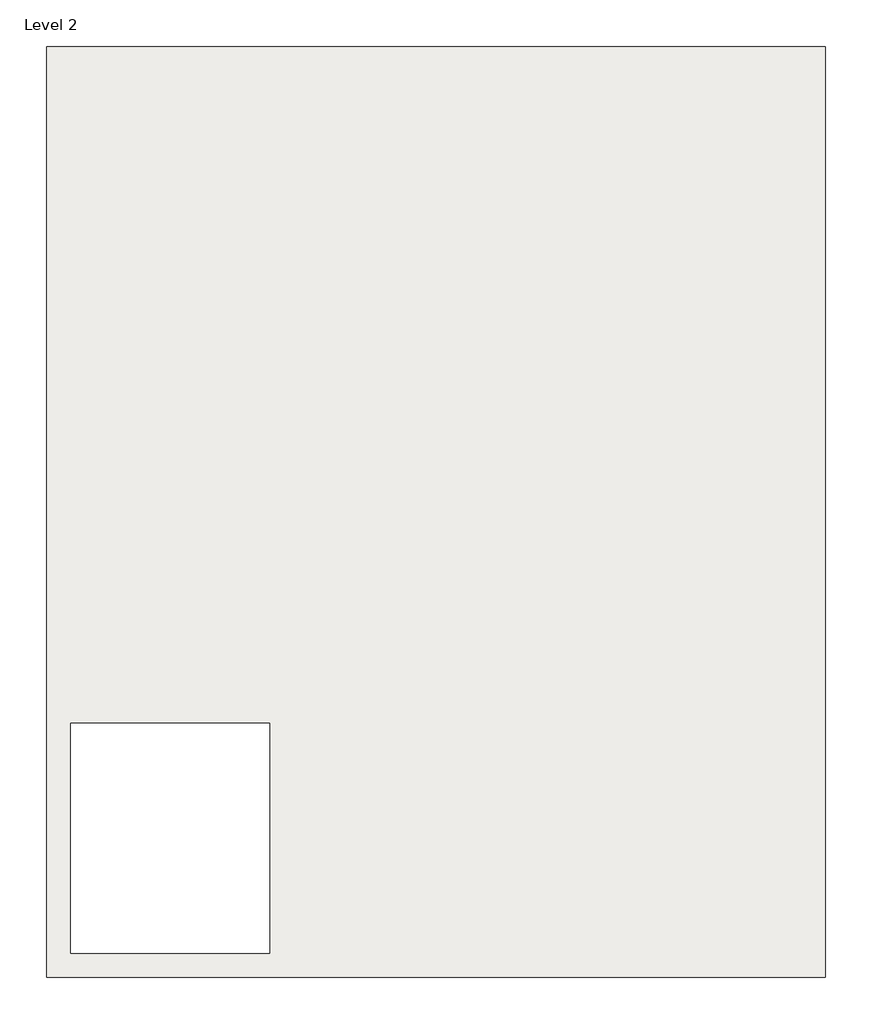
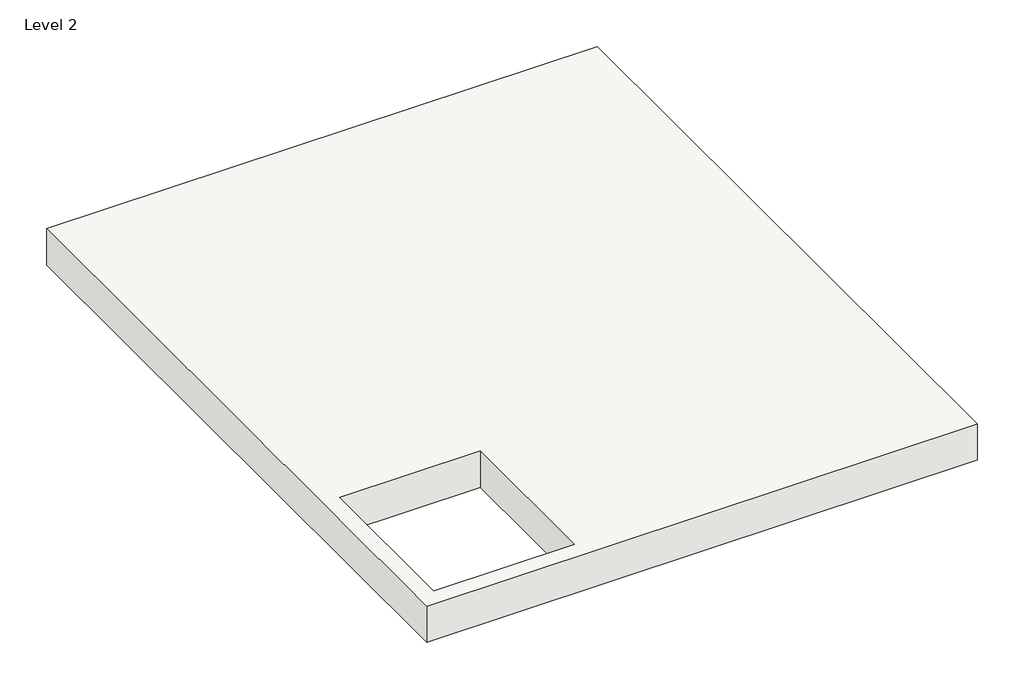
# One storey: 1 roof.
"""IFC4 building model written with IfcOpenShell, lengths in millimetres."""

from ifc_helpers import new_model, si_unit, frame, origin, place, context, project, spatial, polyline, outline, extrude, element, save

model = new_model("IFC4")

# Units and contexts
model_context = context("Model", 3, world=origin())
ifc_project = project(units=[si_unit("LENGTHUNIT", "METRE", prefix="MILLI")], contexts=[model_context])

# Site, building, storey
site = spatial("IfcSite", under=ifc_project)
building = spatial("IfcBuilding", under=site)
storey = spatial("IfcBuildingStorey", under=building, Name="Level 2", Elevation=3048.0)

# Roof
placement = place(None, origin())
element("IfcRoof", 1, ObjectType="Steel Truss - Insulation on Metal Deck - EPDM", at=placement, inside=storey, context=model_context, shape_type="SweptSolid", body=[
    extrude(outline(polyline([(-10104.282173, 13557.9549175), (-2281.082173, 13557.9549175), (-2281.082173, 4210.7549175), (-10104.282173, 4210.7549175), (-10104.282173, 13557.9549175)]), holes=[polyline([(-9863.5624692, 4453.0466042), (-7865.5311534, 4453.0466042), (-7865.5311534, 6764.4466042), (-9863.5624692, 6764.4466042), (-9863.5624692, 4453.0466042)])]), frame((0.0, 0.0, 3048.0), z_axis=(0.0, 0.0, 1.0), x_axis=(1.0, 0.0, 0.0)), (0.0, 0.0, 1.0), 546.1),
])

save(model, "model.ifc")

# Revit data of these elements
# Type "Steel Truss - Insulation on Metal Deck - EPDM"
#   Assembly Code = "B1020"
#   Layers, outside or top first: 0' - 0 1/4" "Roofing, EPDM Membrane" (function 4); 0' - 5" "Rigid insulation" (function 3); 0' - 0 1/4" "Metal Deck" (function 1); 1' - 4" "Structure, Steel Bar Joist Layer" (function 1)
# Element 1 (IfcRoof, "Steel Truss - Insulation on Metal Deck - EPDM")
#   built-in parameter 1001705 = 11.7917 (stored number, unit not read)
#   built-in parameter 1001710 = 33615
#   Phase Created = New Construction
#   Materials on its faces: "Structure, Steel Bar Joist Layer", "Roofing, EPDM Membrane"
# Materials
#   "Roofing, EPDM Membrane": class "Generic", colour RGB 127 127 127, transparency 0, Description = "EPDM roof membrane", Cost = 0
#   "Rigid insulation": class "Generic", colour RGB 127 127 127, transparency 0, Description = "Rigid foam insulation board", Cost = 0
#   "Metal Deck": class "Metal", colour RGB 199 199 199, transparency 0, Description = "Steel, mill finish", Cost = 0
#   "Structure, Steel Bar Joist Layer": class "Metal", colour RGB 127 127 127, transparency 0, Description = "Bar joists, thermal airspace", Cost = 0
